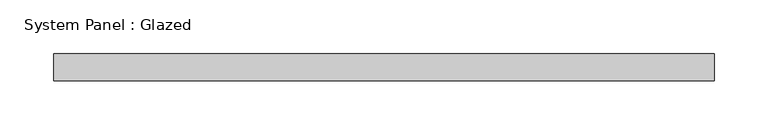
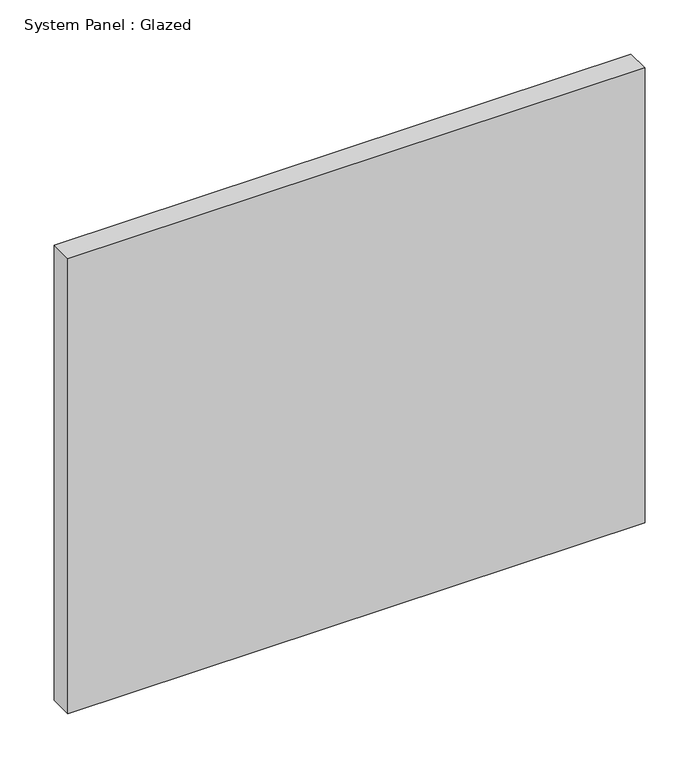
"""IFC4 building model written with IfcOpenShell, lengths in millimetres: plate geometry, System Panel : Glazed."""

from ifc_helpers import new_model, si_unit, origin, origin_with_axes, place, context, project, spatial, polyline, outline, extrude, source, transform, mapped, element, save


def system_panel_glazed_03a03fc4(model_context):
    return source(origin(), model_context, "Body", "SweptSolid", [
        extrude(outline(polyline([(307.975, 19.05), (-307.975, 19.05), (-307.975, 44.45), (307.975, 44.45), (307.975, 19.05)])), origin_with_axes(), (0.0, 0.0, 1.0), 513.3504972),
    ])


if __name__ == "__main__":
    model = new_model("IFC4")
    model_context = context("Model", 3, world=origin())
    ifc_project = project(units=[si_unit("LENGTHUNIT", "METRE", prefix="MILLI")], contexts=[model_context])
    site = spatial("IfcSite", under=ifc_project)
    building = spatial("IfcBuilding", under=site)
    placement = place(None, origin())
    system_panel_glazed_shape = system_panel_glazed_03a03fc4(model_context)
    element("IfcPlate", 1, ObjectType="System Panel : Glazed", at=placement, inside=building, context=model_context, shape_type="MappedRepresentation", body=[
        mapped(system_panel_glazed_shape, transform((0.0, 0.0, 0.0), x_axis=(1.0, 0.0, 0.0), y_axis=(0.0, 1.0, 0.0), z_axis=(0.0, 0.0, 1.0))),
    ])
    save(model, "model.ifc")

# Revit data of these elements
# Type "System Panel : Glazed"
#   Construction Type Id = "GSP4R"
#   Analytic Construction = "1/8 in Pilkington single glazing"
#   Visual Light Transmittance = 0.9
#   Solar Heat Gain Coefficient = 0.86
#   Heat Transfer Coefficient (U) = 1.18115 BTU/(h·ft²·°F)
#   Define Thermal Properties by = 1
# Element 1 (IfcPlate, "System Panel : Glazed")
#   Materials on its faces: "Glass"
# Materials
#   "Glass": class "Glass", colour RGB 0 128 192, transparency 0.75, Description = "Soda Lime Glass", Cost = 0
